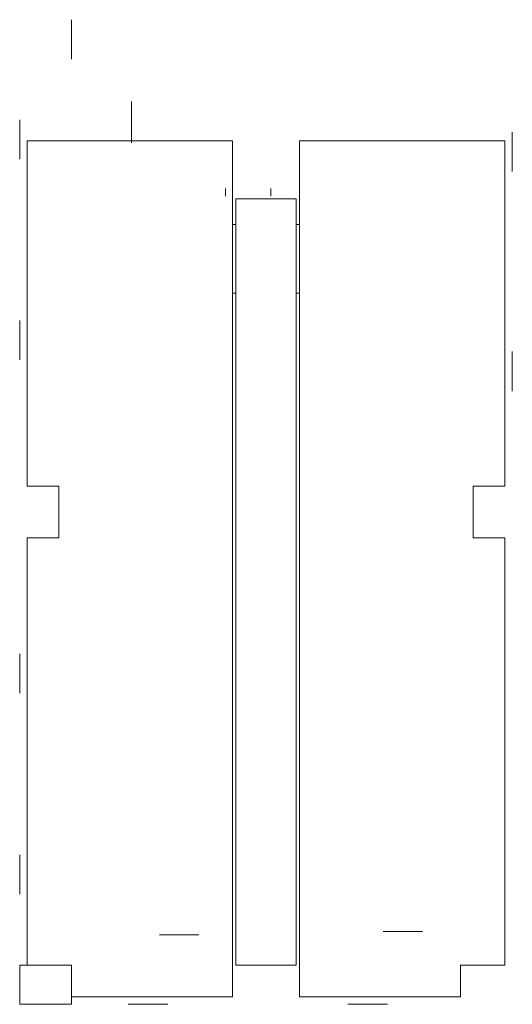
# Model space of a CAD drawing. Units: feet. Extents: x 1080 to 13444, y 870 to 7060.
# Tile 5 of 5: x 12844 to 13444, y 5859 to 7060. Entities that reach past the tile are written whole.
import ezdxf

# ---------------------------------------------------------------- set-up
doc = ezdxf.new("R2010")
doc.units = ezdxf.units.FT
doc.layers.add('A-MODL-LINE', color=8, linetype='Continuous', lineweight=18)

msp = doc.modelspace()

# ---------------------------------------------------------------- linework, layer by layer
at = {"layer": 'A-MODL-LINE'}
for p, q in [((13094.9, 6853.6, -7461.9), (13094.9, 6844.5, -7461.9)), ((13150, 6853.6, -7461.9), (13150, 6844.5, -7461.9)), ((13103.5, 6809.8, -7775.2), (13103.5, 6726.2, -7775.2)), ((13107.5, 6726.2, -7775.2), (13107.5, 6809.8, -7775.2)), ((13180.8, 6809.8, -7775.2), (13180.8, 6726.2, -7775.2)), ((13184.8, 6809.8, -7775.2), (13184.8, 6726.2, -7775.2))]:
    msp.add_line(p, q, dxfattribs=at)
at = {"layer": 'A-MODL-LINE', "elevation": -7775.2}
msp.add_lwpolyline([(13103.5, 6114.8), (13103.5, 5943.8), (13103.5, 5868.2), (12907.1, 5868.2), (12907.1, 5906.8), (12853.1, 5906.8), (12853.1, 6427.7), (12891.7, 6427.7), (12891.7, 6490.7), (12853.1, 6490.7), (12853.1, 6911.8), (12853.1, 6490.7), (12891.7, 6490.7), (12891.7, 6427.7), (12853.1, 6427.7), (12853.1, 5906.8), (12907.1, 5906.8), (12907.1, 5868.2), (13103.5, 5868.2), (13103.5, 6726.2), (13107.5, 6726.2), (13107.5, 5906.8), (13180.8, 5906.8), (13180.8, 6726.2), (13184.8, 6726.2), (13184.8, 5868.2), (13381.1, 5868.2), (13381.1, 5906.8), (13435.1, 5906.8), (13435.1, 6427.7), (13396.5, 6427.7), (13396.5, 6490.7), (13435.1, 6490.7), (13435.1, 6911.8), (13184.8, 6911.8), (13184.8, 6809.8), (13184.8, 6809.8), (13184.8, 6809.8), (13180.8, 6809.8), (13180.8, 6841.2), (13107.5, 6841.2), (13107.5, 6809.8), (13103.5, 6809.8), (13103.5, 6911.8), (12853.1, 6911.8)], dxfattribs=at)
msp.add_lwpolyline([(12907.1, 5906.8), (12844.1, 5906.8), (12844.1, 5859.2), (12907.1, 5859.2)], close=True, dxfattribs=at)
at = {"layer": 'A-MODL-LINE'}
for points in [[(12907.1, 7011.6, -8071.9), (12907.1, 7011.6, -7987.9), (12907.1, 7059.6, -7987.9), (12907.1, 7059.6, -8035.9), (12907.1, 7011.6, -8035.9)], [(12907.1, 7011.6, -8071.9), (12907.1, 7011.6, -7987.9), (12907.1, 7059.6, -7987.9), (12907.1, 7059.6, -8035.9), (12907.1, 7011.6, -8035.9)], [(12907.1, 7011.6, -7944.7), (12907.1, 7011.6, -7860.7), (12907.1, 7059.6, -7860.7), (12907.1, 7059.6, -7908.7), (12907.1, 7011.6, -7908.7)], [(12907.1, 7011.6, -8198.1), (12907.1, 7011.6, -8114.1), (12907.1, 7059.6, -8114.1), (12907.1, 7059.6, -8162.1), (12907.1, 7011.6, -8162.1)], [(12980.3, 6911.8, -8154.2), (12980.3, 6911.8, -8070.2), (12980.3, 6959.8, -8070.2), (12980.3, 6959.8, -8118.2), (12980.3, 6911.8, -8118.2)], [(12980.3, 6909.3, -8155.4), (12980.3, 6909.3, -8071.4), (12980.3, 6957.3, -8071.4), (12980.3, 6957.3, -8119.4), (12980.3, 6909.3, -8119.4)], [(12844.1, 6889.5, -7769.2), (12844.1, 6889.5, -7685.2), (12844.1, 6937.5, -7685.2), (12844.1, 6937.5, -7733.2), (12844.1, 6889.5, -7733.2)], [(12844.1, 6889.5, -7895.2), (12844.1, 6889.5, -7811.2), (12844.1, 6937.5, -7811.2), (12844.1, 6937.5, -7859.2), (12844.1, 6889.5, -7859.2)], [(13444.1, 6874.5, -7895.2), (13444.1, 6874.5, -7811.2), (13444.1, 6922.5, -7811.2), (13444.1, 6922.5, -7859.2), (13444.1, 6874.5, -7859.2)], [(13444.1, 6874.5, -7769.1), (13444.1, 6874.5, -7685.1), (13444.1, 6922.5, -7685.1), (13444.1, 6922.5, -7733.1), (13444.1, 6874.5, -7733.1)], [(12844.1, 6644.8, -7769.2), (12844.1, 6644.8, -7685.2), (12844.1, 6692.8, -7685.2), (12844.1, 6692.8, -7733.2), (12844.1, 6644.8, -7733.2)], [(12844.1, 6644.8, -7895.2), (12844.1, 6644.8, -7811.2), (12844.1, 6692.8, -7811.2), (12844.1, 6692.8, -7859.2), (12844.1, 6644.8, -7859.2)], [(13444.1, 6606.9, -7895.2), (13444.1, 6606.9, -7811.2), (13444.1, 6654.9, -7811.2), (13444.1, 6654.9, -7859.2), (13444.1, 6606.9, -7859.2)], [(13444.1, 6606.9, -7769.1), (13444.1, 6606.9, -7685.1), (13444.1, 6654.9, -7685.1), (13444.1, 6654.9, -7733.1), (13444.1, 6606.9, -7733.1)], [(12844.1, 6238.4, -7769.2), (12844.1, 6238.4, -7685.2), (12844.1, 6286.4, -7685.2), (12844.1, 6286.4, -7733.2), (12844.1, 6238.4, -7733.2)], [(12844.1, 6238.4, -7895.2), (12844.1, 6238.4, -7811.2), (12844.1, 6286.4, -7811.2), (12844.1, 6286.4, -7859.2), (12844.1, 6238.4, -7859.2)], [(12844.1, 5993.6, -7769.2), (12844.1, 5993.6, -7685.2), (12844.1, 6041.6, -7685.2), (12844.1, 6041.6, -7733.2), (12844.1, 5993.6, -7733.2)], [(12844.1, 5993.6, -7895.2), (12844.1, 5993.6, -7811.2), (12844.1, 6041.6, -7811.2), (12844.1, 6041.6, -7859.2), (12844.1, 5993.6, -7859.2)], [(13014.3, 5943.8, -7902.8), (13014.3, 5943.8, -7818.8), (13062.3, 5943.8, -7818.8), (13062.3, 5943.8, -7866.8), (13014.3, 5943.8, -7866.8)], [(13286.7, 5947.8, -7901.2), (13286.7, 5947.8, -7817.2), (13334.7, 5947.8, -7817.2), (13334.7, 5947.8, -7865.2), (13286.7, 5947.8, -7865.2)], [(12976.4, 5859.2, -7895.2), (12976.4, 5859.2, -7811.2), (13024.4, 5859.2, -7811.2), (13024.4, 5859.2, -7859.2), (12976.4, 5859.2, -7859.2)], [(12976.4, 5859.2, -7769.2), (12976.4, 5859.2, -7685.2), (13024.4, 5859.2, -7685.2), (13024.4, 5859.2, -7733.2), (12976.4, 5859.2, -7733.2)], [(13244, 5859.2, -7895.2), (13244, 5859.2, -7811.2), (13292, 5859.2, -7811.2), (13292, 5859.2, -7859.2), (13244, 5859.2, -7859.2)], [(13244, 5859.2, -7769.2), (13244, 5859.2, -7685.2), (13292, 5859.2, -7685.2), (13292, 5859.2, -7733.2), (13244, 5859.2, -7733.2)]]:
    msp.add_polyline3d(points, dxfattribs=at)

doc.saveas('drawing.dxf')
